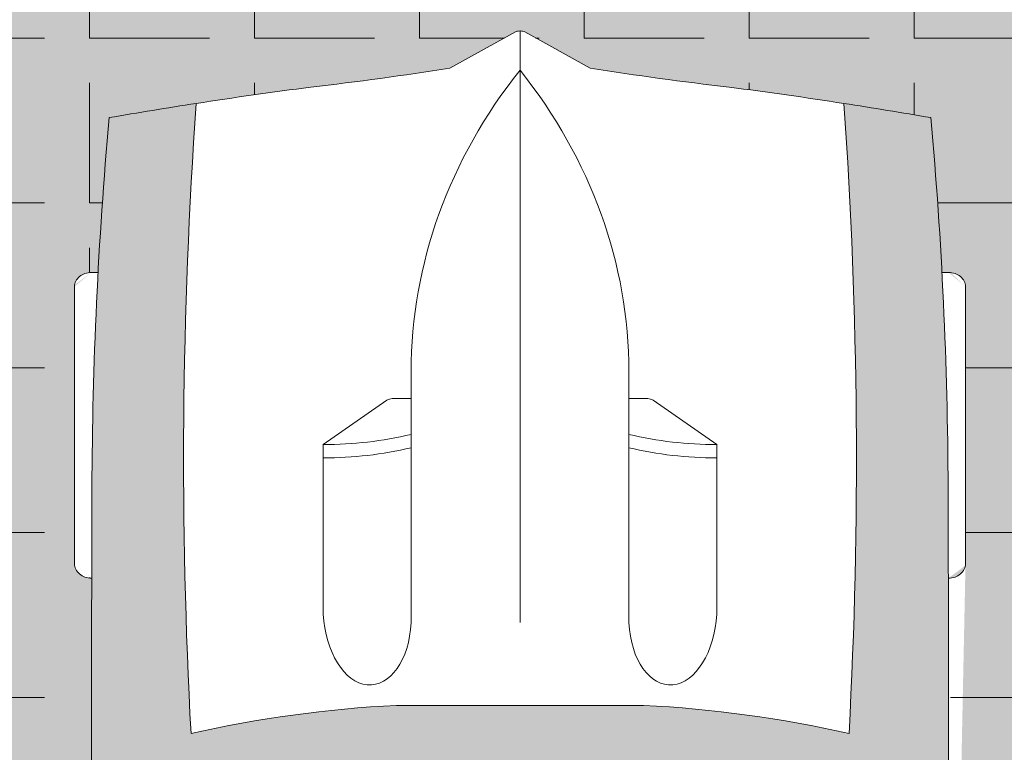
# Model space of a CAD drawing. Units: millimetres. Extents: x 1166 to 16630, y -7192 to 2820.
# Tile 4 of 8: x 5842 to 7051, y -3952 to -3052. Entities that reach past the tile are written whole.
import ezdxf

# ---------------------------------------------------------------- set-up
doc = ezdxf.new("R2010")
doc.units = ezdxf.units.MM
doc.layers.add('A-FLOR-FNSH-PATT', color=254, linetype='Continuous', lineweight=13, true_color=0xfeeab9)
doc.layers.add('C-PKNG-VEHI-PATT', color=18, linetype='Continuous', lineweight=13, true_color=0x000000)
doc.layers.add('A-FLOR-PATT', color=8, linetype='Continuous', lineweight=13)
doc.layers.add('C-PKNG-VEHI', color=8, linetype='Continuous', lineweight=18)

# ---------------------------------------------------------------- blocks, each defined once
blk = doc.blocks.new('*U6')
for p, q in [((46.55368679439944, 38.88847654282876), (22.35054758993934, 38.88847654282876)), ((21.10406751471477, 37.40863046792069), (21.10406751471477, 36.83230215753705)), ((47.80016686962392, 37.39011648242055), (47.80016686962392, 37.40863046792069)), ((32.26591480791686, 11.62530558863241), (36.12873726252356, 17.16961494239206)), ((36.12873726252356, 17.16961494239206), (50.93891189819171, 17.16961494239206)), ((32.12291633764599, 9.505833383620029), (32.12291633764599, 11.15369945057711)), ((58.9167604809788, -10.77488335095668), (58.9167604809788, 10.77488335095617)), ((29.77279020470884, 9.505833383620029), (51.68362801571248, 9.505833383620029)), ((3.266462181856987, 6.128290093440767), (0.1022408397004821, 0.4060708604429806)), ((-4.43e-14, -2.558e-13), (51.68362801571248, -2.558e-13)), ((0.1022408397004821, -0.4060708604432933), (3.266462181856987, -6.128290093441194)), ((29.77279020470884, -9.50583338362054), (51.68362801571248, -9.50583338362054)), ((32.12291633764599, -9.50583338362054), (32.12291633764599, -11.15369945057762)), ((32.26591480791686, -11.62530558863292), (36.12873726252356, -17.16961494239257)), ((36.12873726252356, -17.16961494239257), (50.93891189819171, -17.16961494239257)), ((21.10406751471477, -37.4086304679212), (21.10406751471477, -36.83230215753756)), ((47.80016686962392, -37.39011648242107), (47.80016686962392, -37.4086304679212)), ((46.55368679439944, -38.88847654282927), (22.35054758993934, -38.88847654282927))]:
    blk.add_line(p, q)
for centre, major_axis, ratio, start_param, end_param in [((22.35054758993934, 37.40863046792072), (2.08e-14, -1.479846074908118), 0.842303869543976, 3.141592653589776, 4.712388980384677), ((46.55368679439944, 37.40863046792072), (2.2e-14, 1.479846074908118), 0.8423038695439758, -1.570796326794884, 1.73e-14), ((41.19115208863305, -490.8631038926156), (1.294e-13, 528.2339998381949), 0.8423038695439741, 0.0028100083536837, 0.0755983031096952), ((64.48199294511879, -10555.61767587835), (1.907644e-10, 10593.02630634627), 0.842303869543847, -0.0133969486112073, 0.0027970409639888), ((266.0300214172791, -27.52442688366631), (1.966072e-10, 313.3077612809058), 0.8423038695435284, 1.367075990158062, 1.391760499156098), ((37.47375371777758, -593.9621830607928), (6.21e-14, -623.32820996736), 0.8423038695439826, 3.09604606856106, 3.200911180495224), ((134.4003789125686, 5.387441675477674), (4.276e-13, -89.7774543484738), 0.84230386954398, 4.44948196380473, 4.652344057257214), ((259.1750197310735, -27.52442688366614), (1.506617e-10, -305.3028914627677), 0.8423038695443789, 4.528606069860317, 4.561837674556238), ((-204.4946649195746, 52.39684969293512), (4.12053e-11, -250.9602162198571), 0.8423038695441164, 1.385369446298923, 1.434372047871027), ((13.03653510440275, 17.00972444508943), (1.2303e-12, 27.41599049210566), 0.8423038695439277, 4.435146050259648, 4.718221029521873), ((14.20086229321332, 17.00972444508943), (1.2303e-12, 27.41599049210566), 0.8423038695439277, 4.435146050259648, 4.718221029521873), ((50.7902773840875, 13.33772416300607), (6.340077547122382, -0.356608581037027), 0.6038335755719145, -1.39555193967809, 1.581314658479915), ((32.74615637525823, 11.15369945057713), (1.313e-13, 0.7399230374541176), 0.8423038695439091, 0.8797135699495516, 1.570796326795045), ((29.77279020470884, -46.66302566589627), (5.12e-14, 56.16885904951626), 0.842303869543976, 7e-16, 0.5903187773915901), ((0.6232400376122422, -1.421e-13), (1e-16, -0.7399230374541245), 0.842303869543842, 4.131459131953847, 5.293318828815531), ((29.77279020470884, 46.66302566589578), (4.004e-13, 56.16885904951626), 0.8423038695439734, 2.55127387619821, 3.141592653589801), ((-204.4946649195746, -52.39684969293552), (4.02945e-11, 250.9602162198562), 0.8423038695441192, -1.43437204787103, -1.385369446298926), ((13.03653510440275, -17.00972444508983), (1.2568e-12, -27.41599049210552), 0.8423038695439318, 1.564964277657711, 1.848039256919935), ((14.20086229321332, -17.00972444508983), (1.2568e-12, -27.41599049210552), 0.8423038695439318, 1.564964277657711, 1.848039256919935), ((32.74615637525823, -11.1536994505777), (1.3e-13, -0.7399230374541176), 0.8423038695439093, 4.712388980384541, 5.403471737230034), ((134.4003789125684, -5.387441675478584), (4.2949e-12, -89.77745434847827), 0.8423038695439354, -1.510751403667474, -1.307889310215002), ((259.1750197310694, 27.52442688365929), (1.08535e-11, 305.3028914629043), 0.8423038695439974, 1.721347632622872, 1.754579237318777), ((266.0300214172791, 27.52442688366566), (8.75241e-11, 313.3077612806533), 0.8423038695441819, 1.749832154434603, 1.774516663432659), ((37.47375371777847, 593.9621830607904), (1.1693e-12, -623.3282099673584), 0.8423038695439528, -0.0593185269054384, 0.0455465850287298), ((41.19115208863322, 490.8631038926152), (1.37757e-11, -528.2339998381949), 0.8423038695440652, -0.0755983031097181, -0.0028100083537155), ((64.48199294495228, 10555.61767590795), (6.117947e-10, 10593.02630637587), 0.8423038695458146, 3.138795612625926, 3.154989602201039), ((22.35054758993934, -37.40863046792117), (2.2e-14, 1.479846074908118), 0.8423038695439758, 1.570796326794908, 3.14159265358981), ((46.55368679439944, -37.40863046792117), (2.08e-14, -1.479846074908118), 0.842303869543976, -1.69e-14, 1.570796326794884)]:
    blk.add_ellipse(centre, major_axis=major_axis, ratio=ratio, start_param=start_param, end_param=end_param)
at = {"extrusion": (0, 0, -1)}
blk.add_ellipse((50.7902773840875, -13.33772416300655), major_axis=(6.340077547122382, 0.3566085810370246), ratio=0.6038335755719145, start_param=-1.39555193967809, end_param=1.581314658479915, dxfattribs=at)

msp = doc.modelspace()

# ---------------------------------------------------------------- hatches: boundary and pattern name
at = {"layer": 'A-FLOR-FNSH-PATT', "transparency": 33554590}
h = msp.add_hatch(color=256, dxfattribs=at)
h.dxf.hatch_style = 1
h.paths.add_polyline_path([(5309.614992693758, -2642.53776490782), (5309.614992693758, -6304.141088113749), (7725.939441137629, -6304.141088113749), (7725.939441137629, -5672.53776490782), (7725.939441137629, -2642.53776490782)])
edge = h.paths.add_edge_path(flags=16)
edge.add_ellipse((-448.9724108440159, -3645.429588524165), major_axis=(-7430.722679011307, 2.05049e-10), ratio=0.8423038695440578, start_angle=182.1799503136468, end_angle=183.6504275857006, ccw=False)
edge.add_line((6974.17381326888, -3362.862478220109), (6984.715647929133, -3362.862478220109))
edge.add_ellipse((6982.28108362224, -3380.396843230207), major_axis=(-20.81714882728829, 5.19e-13), ratio=0.842303869543992, start_angle=180.0000000000014, end_angle=270.0000000000014, ccw=False)
edge.add_line((7003.098232449528, -3380.396843230198), (7003.098232449528, -3722.915565549822))
edge.add_ellipse((6982.28108362224, -3720.864922613471), major_axis=(20.81714882728829, 5.097e-13), ratio=0.842303869543992, start_angle=269.9999999999985, end_angle=359.9999999999986, ccw=False)
edge.add_ellipse((-142030.922985108, -3973.064272051784), major_axis=(149013.2040687302, 7.3876543e-09), ratio=0.8423038695454406, start_angle=-0.3838667787953227, end_angle=0.09022908859151357, ccw=False)
edge.add_line((6977.567346638728, -4971.397229994678), (6984.470063297348, -4971.397229994678))
edge.add_ellipse((6982.28108362224, -4988.931595004776), major_axis=(20.81714882728829, 5.4695e-12), ratio=0.84230386954397, start_angle=-1.5006662579253316e-11, end_angle=89.99999999998488, ccw=False)
edge.add_line((7003.098232449528, -4988.931595004766), (7003.098232449527, -5331.243460438734))
edge.add_ellipse((6982.281083622239, -5329.399674388036), major_axis=(-20.81714882728829, 1.0505e-12), ratio=0.84230386954397, start_angle=90.0000000000029, end_angle=180.000000000003, ccw=False)
edge.add_line((6982.281083622243, -5346.934039398132), (6973.353954790083, -5346.934039398132))
edge.add_ellipse((-142030.922985108, -3973.064272051784), major_axis=(149013.2040687302, 7.3876543e-09), ratio=0.8423038695454406, start_angle=-0.6186431963221253, end_angle=-0.5282714718208013, ccw=False)
edge.add_ellipse((6960.189207408767, -5606.902802775503), major_axis=(-31.22572324093233, 2.0889e-12), ratio=0.8423038695439425, start_angle=179.3717627838109, end_angle=248.4647566010108, ccw=False)
edge.add_ellipse((-142041.331559525, -3973.064272085929), major_axis=(-149045.3717863939, 4.64621177404e-05), ratio=0.8423038661083152, start_angle=179.3534459208122, end_angle=179.3717628016453, ccw=False)
edge.add_ellipse((6916.869834512962, -5654.054118847628), major_axis=(-73.80201542105252, 3.6097e-12), ratio=0.8423038695439748, start_angle=90.00000000006492, end_angle=179.353445902922, ccw=False)
edge.add_line((6916.869834513031, -5716.217842016925), (5995.230132669023, -5716.217842016909))
edge.add_ellipse((5995.230132669163, -5654.054118847574), major_axis=(73.80201542109666, 3.978e-13), ratio=0.8423038695439887, start_angle=180.6465540970575, end_angle=269.9999999998622, ccw=False)
edge.add_ellipse((154953.4315273228, -3973.06427200764), major_axis=(-149045.3717871212, 2.2898328512e-06), ratio=0.8423038697262194, start_angle=0.6282372171232851, end_angle=0.6465540979564253, ccw=False)
edge.add_ellipse((5951.910759773294, -5606.902802775455), major_axis=(31.22572324094488, 4.9039e-12), ratio=0.842303869543988, start_angle=111.53524350401449, end_angle=180.6282372161637, ccw=False)
edge.add_ellipse((154943.0229527065, -3973.064272049507), major_axis=(-149013.2040691466, 7.4869171e-09), ratio=0.8423038695459824, start_angle=0.528271471820176, end_angle=0.6465540970638131, ccw=False)
edge.add_line((5938.746012391977, -5346.934039398132), (5927.384319252956, -5346.934039398132))
edge.add_ellipse((5929.818883559845, -5329.399674388033), major_axis=(20.8171488272892, 3.11e-13), ratio=0.8423038695440205, start_angle=179.9999999999992, end_angle=269.9999999999962, ccw=False)
edge.add_line((5909.001734732555, -5329.399674388034), (5909.001734732554, -4986.88095206843))
edge.add_ellipse((5929.818883559843, -4988.931595004776), major_axis=(-20.8171488272892, 3.063e-13), ratio=0.8423038695440205, start_angle=-89.99999999999608, end_angle=7.958078640513122e-13, ccw=False)
edge.add_line((5929.818883559843, -4971.397229994676), (5934.53262054336, -4971.397229994676))
edge.add_ellipse((154943.0229527065, -3973.064272049507), major_axis=(-149013.2040691466, 7.4869171e-09), ratio=0.8423038695459824, start_angle=-0.09022908859031986, end_angle=0.38386677879520903, ccw=False)
edge.add_ellipse((5929.818883559843, -3720.864922613471), major_axis=(-20.8171488272892, 1.5867e-12), ratio=0.8423038695439331, start_angle=4.376943252282217e-12, end_angle=90.00000000000438, ccw=False)
edge.add_line((5909.001734732555, -3720.864922613478), (5909.001734732555, -3378.346200293855))
edge.add_ellipse((5929.818883559843, -3380.396843230207), major_axis=(20.8171488272892, 9.396e-13), ratio=0.8423038695439548, start_angle=89.99999999999739, end_angle=179.9999999999975, ccw=False)
edge.add_line((5929.818883559843, -3362.862478220109), (5937.926153913206, -3362.862478220109))
edge.add_ellipse((13361.0723780261, -3645.42958852417), major_axis=(7430.722679011307, 7.96527e-11), ratio=0.8423038695440075, start_angle=176.3495724143003, end_angle=177.8200496863542, ccw=False)
edge.add_ellipse((6843.238962592569, -6808.26137511002), major_axis=(4407.332901654202, 4.993684e-10), ratio=0.8423038695438785, start_angle=102.12596555227748, end_angle=103.7805289894913, ccw=False)
edge.add_ellipse((6843.238962592481, -6711.831352601092), major_axis=(4294.727564406183, 8.108409e-10), ratio=0.8423038695438188, start_angle=100.20953899713243, end_angle=102.4446272934332, ccw=False)
edge.add_ellipse((5718.978043047074, -189.3416182050969), major_axis=(-3530.283493235897, 2.29487e-11), ratio=0.8423038695439934, start_angle=99.25656600720184, end_angle=102.5549326441376)
edge.add_line((6369.842688727707, -3111.939026631001), (6452.046781461999, -3066.482546539763))
edge.add_ellipse((6456.049983591043, -3074.756545497792), major_axis=(-10.40857441364578, 1.5838e-12), ratio=0.8423038695437935, start_angle=270.0000000000206, end_angle=307.9331304598557, ccw=False)
edge.add_ellipse((6456.049983591043, -3074.756545497792), major_axis=(-10.40857441364578, 1.5838e-12), ratio=0.8423038695437935, start_angle=232.06686954016618, end_angle=270.0000000000206, ccw=False)
edge.add_line((6461.762224667734, -3067.427595530816), (6542.257278454378, -3111.939026631002))
edge.add_ellipse((7193.121924135012, -189.3416182050969), major_axis=(3530.283493235459, 5.426614e-10), ratio=0.842303869544094, start_angle=257.4450673558539, end_angle=260.7434339927895)
edge.add_ellipse((6068.861004589511, -6711.831352601148), major_axis=(4294.72756440461, 7.517164e-10), ratio=0.8423038695441345, start_angle=77.55537270654469, end_angle=79.79046100284552, ccw=False)
edge.add_ellipse((6068.86100458951, -6808.26137511002), major_axis=(-4407.332901654327, 6.637773e-10), ratio=0.842303869543856, start_angle=256.2194710105107, end_angle=257.8740344477245, ccw=False)
edge = h.paths.add_edge_path(flags=0)
edge.add_ellipse((5799.636342679871, -3484.80630294614), major_axis=(790.1331889300527, 2.1537e-12), ratio=0.8423038695439757, start_angle=-2.2737367544323206e-13, end_angle=29.43856959797921, ccw=False)
edge.add_line((6589.769531609924, -3484.806302946152), (6589.769531609924, -3517.865771969153))
edge.add_line((6589.769531609924, -3517.865771969153), (6615.396946753699, -3517.865771969153))
edge.add_ellipse((6612.950235160742, -3526.632954474201), major_axis=(10.40857441364348, 1.5653e-12), ratio=0.8423038695440233, start_angle=45.51978911742219, end_angle=89.99999999999147, ccw=False)
edge.add_line((6619.58436781158, -3519.877346340421), (6697.576744801804, -3574.216072032502))
edge.add_line((6697.576744801804, -3574.216072032502), (6697.576744801804, -3782.552340767745))
edge.add_ellipse((6643.673138205864, -3780.461483581003), major_axis=(5.016450041930374, 89.18653102701357), ratio=0.6038335755719256, start_angle=106.34259195429391, end_angle=270.99798572497, ccw=False)
edge.add_line((6589.769531609924, -3793.028339937766), (6589.769531609924, -3484.806302946153))
edge.add_ellipse((5799.636342679871, -3484.80630294614), major_axis=(790.1331889300527, 2.1537e-12), ratio=0.8423038695439757, start_angle=-2.143e-13, end_angle=29.43856959797918)
edge.add_ellipse((7112.463624502211, -3484.80630294614), major_axis=(-790.1331889300524, 7.9434e-12), ratio=0.8423038695439707, start_angle=-29.43856959797882, end_angle=5.465e-13)
edge.add_line((6322.330435572158, -3484.806302946151), (6322.330435572158, -3793.028339937766))
edge.add_ellipse((6268.426828976219, -3780.461483581003), major_axis=(-5.016450041930374, 89.18653102701357), ratio=0.6038335755719256, start_angle=89.00201427502998, end_angle=253.6574080457062, ccw=False)
edge.add_line((6214.523222380278, -3782.552340767737), (6214.523222380279, -3574.216072032502))
edge.add_line((6214.523222380279, -3574.216072032502), (6294.400928520307, -3518.563802793423))
edge.add_ellipse((6299.149732021341, -3526.632954474201), major_axis=(10.4085744136453, 3.381e-13), ratio=0.8423038695438764, start_angle=89.9999999999983, end_angle=134.4802108825654, ccw=False)
edge.add_line((6299.149732021338, -3517.865771969152), (6322.330435572158, -3517.865771969152))
edge.add_line((6322.330435572158, -3517.865771969152), (6322.330435572158, -3484.806302946154))
edge.add_ellipse((7112.463624502211, -3484.80630294614), major_axis=(-790.1331889300524, 7.9434e-12), ratio=0.8423038695439707, start_angle=-29.438569597978812, end_angle=6.252776074688882e-13, ccw=False)
edge = h.paths.add_edge_path(flags=0)
edge.add_line((6899.672020630411, -4051.112638739672), (6868.937058315451, -4281.473694083312))
edge.add_ellipse((6495.430033257824, -5170.362894493258), major_axis=(1119.455420763322, 3.0514e-12), ratio=0.8423038695439744, start_angle=67.20808512240981, end_angle=85.12993040286408)
edge.add_line((6575.564661792019, -4229.860228440724), (6336.53530539007, -4229.860228440724))
edge.add_ellipse((6416.669933924288, -5170.362894493482), major_axis=(1119.455420763633, 5.82337e-11), ratio=0.842303869543943, start_angle=94.87006959713275, end_angle=112.7919148775836)
edge.add_line((6043.162908866626, -4281.473694083309), (6012.427946551666, -4051.112638739666))
edge.add_ellipse((6380.264280565288, -4969.144446445703), major_axis=(1150.303461305961, 5.9583e-11), ratio=0.8423038695439412, start_angle=94.27742096305099, end_angle=111.83495379670521, ccw=False)
edge.add_line((6307.939299228742, -4002.156437400477), (6604.160667953341, -4002.156437400477))
edge.add_ellipse((6531.835686616772, -4969.144446445682), major_axis=(-1150.303461305901, 2.25473e-11), ratio=0.8423038695439672, start_angle=248.1650462032914, end_angle=265.72257903694555, ccw=False)
edge = h.paths.add_edge_path(flags=0)
edge.add_ellipse((-142030.9229855244, -3973.064272050007), major_axis=(-148992.3869203194, 2.076209e-10), ratio=0.842303869544003, start_angle=179.6222358060902, end_angle=179.9444056865007, ccw=False)
edge.add_line((6956.899516505626, -4955.389335168179), (6903.06848209712, -4744.029778632651))
edge.add_ellipse((-45118.92430422086, -4413.460367112857), major_axis=(52023.47313689829, 7.771381e-10), ratio=0.842303869543516, start_angle=-0.3640763488911976, end_angle=0.1208973690317991)
edge.add_line((6904.3855953652, -4303.688047353878), (6961.365076797346, -4117.63210307358))
edge = h.paths.add_edge_path(flags=0)
edge.add_line((5950.734890384741, -4117.632103073563), (6007.714371816899, -4303.688047353918))
edge.add_ellipse((58031.02427140294, -4413.460367113082), major_axis=(-52023.47313689826, 1.3200601e-09), ratio=0.8423038695497072, start_angle=-0.1208973690315197, end_angle=0.364076348891516)
edge.add_line((6009.031485084967, -4744.029778632643), (5955.200450676423, -4955.389335168309))
edge.add_ellipse((154943.0229527063, -3973.064272050686), major_axis=(-148992.3869203192, 3.28274152e-08), ratio=0.8423038695536886, start_angle=0.05559431351167632, end_angle=0.3777641939223031, ccw=False)
edge = h.paths.add_edge_path(flags=0)
edge.add_line((6868.937058315452, -5013.198477251068), (6868.937058315452, -5277.993200767081))
edge.add_ellipse((6456.049983591043, -3571.079447459644), major_axis=(2068.11644385622, 7.9333e-12), ratio=0.8423038695439821, start_angle=256.4018653097692, end_angle=283.59813469023027, ccw=False)
edge.add_line((6043.16290886663, -5277.993200767081), (6043.16290886663, -5013.198477251068))
edge.add_ellipse((6456.049983591043, -3306.284723943631), major_axis=(2068.116443856253, 3.3411e-12), ratio=0.8423038695439679, start_angle=256.4018653097692, end_angle=283.5981346902304)
edge = h.paths.add_edge_path(flags=0)
edge.add_ellipse((6827.302760660877, -5415.313265203762), major_axis=(-41.63429765457658, 1.038e-12), ratio=0.842303869543992, start_angle=180.0000000000014, end_angle=270.0000000000014, ccw=False)
edge.add_line((6868.937058315454, -5415.313265203762), (6868.937058315454, -5689.12284886784))
edge.add_line((6868.937058315454, -5689.12284886784), (6043.162908866631, -5689.122848867824))
edge.add_line((6043.162908866631, -5689.122848867824), (6043.16290886663, -5415.313265203758))
edge.add_ellipse((6084.797206521206, -5415.313265203759), major_axis=(-41.63429765457658, 3.4138e-12), ratio=0.842303869543992, start_angle=-89.99999999999523, end_angle=4.718003765447065e-12, ccw=False)
edge.add_line((6084.797206521207, -5380.244535183563), (6827.302760660879, -5380.244535183566))
h.paths.add_polyline_path([(3455.939441137629, -522.53776490782), (1955.939441137629, -522.53776490782), (1955.939441137629, -2522.53776490782), (3455.939441137629, -2522.53776490782), (3455.939441137628, -2456.640093510054), (2713.439441137629, -2456.640093510054), (2713.43944113763, -2423.827593510054), (2714.157558370035, -2423.827593510054, -0.398552660000795), (3455.939441137629, -1706.6775944476)])
h.paths.add_polyline_path([(2617.666699633915, -1084.404517764245, -0.1328909081885223), (2584.2707950462, -1084.404517500826, -0.5013167773008519), (2505.064916213601, -782.9330743979599), (2537.033121160981, -687.0284595558127), (2489.081652205778, -687.0284595558132), (2489.081652205778, -711.0041940334158), (2441.130183250573, -711.0041940334158), (2441.130183250573, -695.0203710483474), (2473.097829220709, -695.0203710483474), (2473.097829220709, -687.0284595558132), (2433.13827175804, -687.0284595558132), (2433.138271758038, -559.1578756752674), (2768.79855444447, -559.1578756752674), (2768.798554444471, -687.0284595558132), (2664.903705041528, -687.0284595558132), (2696.870765296628, -782.9296403211174, -0.5013234908365807)], flags=16)
h.paths.add_polyline_path([(2627.246667254758, -1063.015793855155, -0.2150037826753064), (2574.690827957319, -1063.015793301825, -0.4800796505537303), (2537.033991046725, -782.9313974662227), (2664.904416594217, -782.9313974662227, -0.4800795019660876)], flags=0)
h.paths.add_polyline_path([(2736.830905816404, -671.0446365707452), (2465.105920386107, -671.0446365707452, -0.5000001164022092), (2449.122094743107, -655.0608109277463), (2449.122094743107, -591.1255243033341, -0.5000001164022404), (2465.105920386111, -575.1416986603361), (2736.830905816402, -575.1416986603361, -0.5000001164023353), (2752.814731459403, -591.1255243033406), (2752.814731459403, -655.0608109277468, -0.50000011640211)], flags=0)
h.paths.add_polyline_path([(5931.781743219382, -6111.826019846759), (7070.309755611069, -6111.826019846759), (7070.309755611069, -5852.301891921869), (5931.781743219382, -5852.301891921869)], flags=24)
h.paths.add_polyline_path([(2102.335631979146, -1543.656328414819), (3007.075088498303, -1543.656328414819), (3007.075088498303, -1283.961010431932), (2102.335631979146, -1283.961010431932)], flags=24)
at = {"layer": 'A-FLOR-PATT', "transparency": 33554564}
h = msp.add_hatch(dxfattribs=at)
h.set_pattern_fill('ANGLE', color=256, scale=29)
h.set_pattern_definition([(0, (-8657.519420588213, -11987.85165359825), (0, 202.565), [147.32, -55.24499999999999]), (90, (-8657.519420588213, -11987.85165359825), (-202.565, 1.24e-14), [147.32, -55.24499999999999])])
h.paths.add_polyline_path([(7725.939441137629, -2642.53776490782), (5309.614992693758, -2642.53776490782), (5309.614992693758, -6304.141088113749), (7725.939441137629, -6304.141088113749), (7725.939441137629, -5672.53776490782)])
edge = h.paths.add_edge_path(flags=16)
edge.add_ellipse((-142030.922985108, -3973.064272051784), major_axis=(149013.2040687302, 7.3876543e-09), ratio=0.8423038695454406, start_angle=-0.3838667787953227, end_angle=0.09022908859151357, ccw=False)
edge.add_ellipse((6982.28108362224, -4988.931595004776), major_axis=(20.81714882728829, 5.4695e-12), ratio=0.84230386954397, start_angle=-1.5006662579253316e-11, end_angle=89.99999999998488, ccw=False)
edge.add_line((7003.098232449528, -4988.931595004773), (7003.098232449527, -5329.399674388036))
edge.add_ellipse((6982.281083622239, -5329.399674388036), major_axis=(-20.81714882728829, 1.0505e-12), ratio=0.84230386954397, start_angle=90.0000000000029, end_angle=180.000000000003, ccw=False)
edge.add_line((6982.281083622241, -5346.934039398132), (6973.353954790083, -5346.934039398132))
edge.add_ellipse((-142030.922985108, -3973.064272051784), major_axis=(149013.2040687302, 7.3876543e-09), ratio=0.8423038695454406, start_angle=-0.6186431963221253, end_angle=-0.5282714718208013, ccw=False)
edge.add_ellipse((6960.189207408767, -5606.902802775503), major_axis=(-31.22572324093233, 2.0889e-12), ratio=0.8423038695439425, start_angle=179.3717627838109, end_angle=248.4647566010108, ccw=False)
edge.add_ellipse((-142041.331559525, -3973.064272085929), major_axis=(-149045.3717863939, 4.64621177404e-05), ratio=0.8423038661083152, start_angle=179.3534459208122, end_angle=179.3717628016453, ccw=False)
edge.add_ellipse((6916.869834512962, -5654.054118847628), major_axis=(-73.80201542105252, 3.6097e-12), ratio=0.8423038695439748, start_angle=90.00000000006492, end_angle=179.353445902922, ccw=False)
edge.add_line((6916.869834513029, -5716.217842016925), (5995.230132669016, -5716.217842016909))
edge.add_ellipse((5995.230132669163, -5654.054118847574), major_axis=(73.80201542109666, 3.978e-13), ratio=0.8423038695439887, start_angle=180.6465540970575, end_angle=269.9999999998622, ccw=False)
edge.add_ellipse((154953.4315273228, -3973.06427200764), major_axis=(-149045.3717871212, 2.2898328512e-06), ratio=0.8423038697262194, start_angle=0.6282372171232851, end_angle=0.6465540979564253, ccw=False)
edge.add_ellipse((5951.910759773294, -5606.902802775455), major_axis=(31.22572324094488, 4.9039e-12), ratio=0.842303869543988, start_angle=111.53524350401449, end_angle=180.6282372161637, ccw=False)
edge.add_ellipse((154943.0229527065, -3973.064272049507), major_axis=(-149013.2040691466, 7.4869171e-09), ratio=0.8423038695459824, start_angle=0.528271471820176, end_angle=0.6465540970638131, ccw=False)
edge.add_line((5938.746012391977, -5346.934039398132), (5929.818883559843, -5346.934039398132))
edge.add_ellipse((5929.818883559845, -5329.399674388033), major_axis=(20.8171488272892, 3.11e-13), ratio=0.8423038695440205, start_angle=179.9999999999992, end_angle=269.9999999999962, ccw=False)
edge.add_line((5909.001734732555, -5329.399674388033), (5909.001734732554, -4988.931595004778))
edge.add_ellipse((5929.818883559843, -4988.931595004776), major_axis=(-20.8171488272892, 3.063e-13), ratio=0.8423038695440205, start_angle=-89.99999999999608, end_angle=7.958078640513122e-13, ccw=False)
edge.add_ellipse((154943.0229527065, -3973.064272049507), major_axis=(-149013.2040691466, 7.4869171e-09), ratio=0.8423038695459824, start_angle=-0.09022908859031986, end_angle=0.38386677879520903, ccw=False)
edge.add_ellipse((5929.818883559843, -3720.864922613471), major_axis=(-20.8171488272892, 1.5867e-12), ratio=0.8423038695439331, start_angle=4.376943252282217e-12, end_angle=90.00000000000438, ccw=False)
edge.add_line((5909.001734732555, -3720.864922613472), (5909.001734732555, -3380.396843230204))
edge.add_ellipse((5929.818883559843, -3380.396843230207), major_axis=(20.8171488272892, 9.396e-13), ratio=0.8423038695439548, start_angle=89.99999999999739, end_angle=179.9999999999975, ccw=False)
edge.add_line((5929.818883559843, -3362.862478220109), (5937.926153913207, -3362.862478220109))
edge.add_ellipse((13361.0723780261, -3645.42958852417), major_axis=(7430.722679011307, 7.96527e-11), ratio=0.8423038695440075, start_angle=176.3495724143003, end_angle=177.8200496863542, ccw=False)
edge.add_ellipse((6843.238962592569, -6808.26137511002), major_axis=(4407.332901654202, 4.993684e-10), ratio=0.8423038695438785, start_angle=102.12596555227748, end_angle=103.7805289894913, ccw=False)
edge.add_ellipse((6843.238962592481, -6711.831352601092), major_axis=(4294.727564406183, 8.108409e-10), ratio=0.8423038695438188, start_angle=100.20953899713243, end_angle=102.4446272934332, ccw=False)
edge.add_ellipse((5718.978043047074, -189.3416182050969), major_axis=(-3530.283493235897, 2.29487e-11), ratio=0.8423038695439934, start_angle=99.25656600720184, end_angle=102.5549326441376)
edge.add_line((6369.842688727707, -3111.939026631), (6453.505541262713, -3065.675894661087))
edge.add_ellipse((6456.049983591043, -3074.756545497792), major_axis=(-10.40857441364578, 1.5838e-12), ratio=0.8423038695437935, start_angle=232.06686954016618, end_angle=270.0000000000206, ccw=False)
edge.add_line((6460.053185720086, -3066.482546539763), (6542.257278454378, -3111.939026631002))
edge.add_ellipse((7193.121924135012, -189.3416182050969), major_axis=(3530.283493235459, 5.426614e-10), ratio=0.842303869544094, start_angle=257.4450673558539, end_angle=260.7434339927895)
edge.add_ellipse((6068.861004589511, -6711.831352601148), major_axis=(4294.72756440461, 7.517164e-10), ratio=0.8423038695441345, start_angle=77.55537270654469, end_angle=79.79046100284552, ccw=False)
edge.add_ellipse((6068.86100458951, -6808.26137511002), major_axis=(-4407.332901654327, 6.637773e-10), ratio=0.842303869543856, start_angle=256.2194710105107, end_angle=257.8740344477245, ccw=False)
edge.add_ellipse((-448.9724108440159, -3645.429588524165), major_axis=(-7430.722679011307, 2.05049e-10), ratio=0.8423038695440578, start_angle=182.1799503136468, end_angle=183.6504275857006, ccw=False)
edge.add_line((6974.17381326888, -3362.862478220109), (6982.28108362224, -3362.862478220109))
edge.add_ellipse((6982.28108362224, -3380.396843230207), major_axis=(-20.81714882728829, 5.19e-13), ratio=0.842303869543992, start_angle=180.0000000000014, end_angle=270.0000000000014, ccw=False)
edge.add_line((7003.098232449528, -3380.396843230204), (7003.098232449528, -3720.864922613474))
edge.add_ellipse((6982.28108362224, -3720.864922613471), major_axis=(20.81714882728829, 5.097e-13), ratio=0.842303869543992, start_angle=269.9999999999985, end_angle=359.9999999999986, ccw=False)
edge = h.paths.add_edge_path(flags=0)
edge.add_ellipse((-142030.9229855244, -3973.064272050007), major_axis=(-148992.3869203194, 2.076209e-10), ratio=0.842303869544003, start_angle=179.6222358060902, end_angle=179.9444056865007, ccw=False)
edge.add_line((6956.899516505626, -4955.389335168179), (6903.06848209712, -4744.029778632651))
edge.add_ellipse((-45118.92430422086, -4413.460367112857), major_axis=(52023.47313689829, 7.771381e-10), ratio=0.842303869543516, start_angle=-0.3640763488911976, end_angle=0.1208973690317991)
edge.add_line((6904.3855953652, -4303.688047353878), (6961.365076797346, -4117.632103073563))
edge = h.paths.add_edge_path(flags=0)
edge.add_line((6899.672020630411, -4051.112638739673), (6868.937058315451, -4281.473694083312))
edge.add_ellipse((6495.430033257824, -5170.362894493258), major_axis=(1119.455420763322, 3.0514e-12), ratio=0.8423038695439744, start_angle=67.20808512240981, end_angle=85.12993040286408)
edge.add_line((6575.564661792022, -4229.860228440724), (6336.535305390071, -4229.860228440724))
edge.add_ellipse((6416.669933924288, -5170.362894493482), major_axis=(1119.455420763633, 5.82337e-11), ratio=0.842303869543943, start_angle=94.87006959713275, end_angle=112.7919148775836)
edge.add_line((6043.162908866626, -4281.473694083308), (6012.427946551666, -4051.112638739666))
edge.add_ellipse((6380.264280565288, -4969.144446445703), major_axis=(1150.303461305961, 5.9583e-11), ratio=0.8423038695439412, start_angle=94.27742096305099, end_angle=111.83495379670521, ccw=False)
edge.add_line((6307.939299228742, -4002.156437400477), (6604.16066795334, -4002.156437400477))
edge.add_ellipse((6531.835686616772, -4969.144446445682), major_axis=(-1150.303461305901, 2.25473e-11), ratio=0.8423038695439672, start_angle=248.1650462032914, end_angle=265.72257903694555, ccw=False)
edge = h.paths.add_edge_path(flags=0)
edge.add_ellipse((6643.673138205864, -3780.461483581003), major_axis=(5.016450041930374, 89.18653102701357), ratio=0.6038335755719256, start_angle=106.34259195429391, end_angle=270.99798572497, ccw=False)
edge.add_line((6589.769531609924, -3793.028339937766), (6589.769531609924, -3484.806302946154))
edge.add_ellipse((5799.636342679871, -3484.80630294614), major_axis=(790.1331889300527, 2.1537e-12), ratio=0.8423038695439757, start_angle=-2.143e-13, end_angle=29.43856959797918)
edge.add_ellipse((7112.463624502211, -3484.80630294614), major_axis=(-790.1331889300524, 7.9434e-12), ratio=0.8423038695439707, start_angle=-29.43856959797882, end_angle=5.465e-13)
edge.add_line((6322.330435572158, -3484.806302946151), (6322.330435572158, -3793.028339937766))
edge.add_ellipse((6268.426828976219, -3780.461483581003), major_axis=(-5.016450041930374, 89.18653102701357), ratio=0.6038335755719256, start_angle=89.00201427502998, end_angle=253.6574080457062, ccw=False)
edge.add_line((6214.523222380278, -3782.552340767735), (6214.523222380279, -3574.216072032502))
edge.add_line((6214.523222380279, -3574.216072032502), (6295.402812213822, -3517.865771969152))
edge.add_line((6295.402812213822, -3517.865771969152), (6322.330435572158, -3517.865771969152))
edge.add_line((6322.330435572158, -3517.865771969152), (6322.330435572158, -3484.806302946154))
edge.add_ellipse((7112.463624502211, -3484.80630294614), major_axis=(-790.1331889300524, 7.9434e-12), ratio=0.8423038695439707, start_angle=-29.438569597978812, end_angle=6.252776074688882e-13, ccw=False)
edge.add_ellipse((5799.636342679871, -3484.80630294614), major_axis=(790.1331889300527, 2.1537e-12), ratio=0.8423038695439757, start_angle=-2.2737367544323206e-13, end_angle=29.43856959797921, ccw=False)
edge.add_line((6589.769531609924, -3484.806302946153), (6589.769531609924, -3517.865771969153))
edge.add_line((6589.769531609924, -3517.865771969153), (6616.697154968261, -3517.865771969153))
edge.add_line((6616.697154968261, -3517.865771969153), (6697.576744801804, -3574.216072032502))
edge.add_line((6697.576744801804, -3574.216072032502), (6697.576744801804, -3782.552340767746))
edge = h.paths.add_edge_path(flags=0)
edge.add_line((6868.937058315452, -5013.198477251068), (6868.937058315452, -5277.993200767081))
edge.add_ellipse((6456.049983591043, -3571.079447459644), major_axis=(2068.11644385622, 7.9333e-12), ratio=0.8423038695439821, start_angle=256.4018653097692, end_angle=283.59813469023027, ccw=False)
edge.add_line((6043.16290886663, -5277.993200767081), (6043.16290886663, -5013.198477251067))
edge.add_ellipse((6456.049983591043, -3306.284723943631), major_axis=(2068.116443856253, 3.3411e-12), ratio=0.8423038695439679, start_angle=256.4018653097692, end_angle=283.5981346902304)
edge = h.paths.add_edge_path(flags=0)
edge.add_ellipse((58031.02427140294, -4413.460367113082), major_axis=(-52023.47313689826, 1.3200601e-09), ratio=0.8423038695497072, start_angle=-0.1208973690315197, end_angle=0.364076348891516)
edge.add_line((6009.031485084967, -4744.029778632643), (5955.200450676423, -4955.389335168309))
edge.add_ellipse((154943.0229527063, -3973.064272050686), major_axis=(-148992.3869203192, 3.28274152e-08), ratio=0.8423038695536886, start_angle=0.05559431351167632, end_angle=0.3777641939223031, ccw=False)
edge.add_line((5950.734890384742, -4117.632103073569), (6007.714371816899, -4303.688047353918))
edge = h.paths.add_edge_path(flags=0)
edge.add_ellipse((6827.302760660877, -5415.313265203762), major_axis=(-41.63429765457658, 1.038e-12), ratio=0.842303869543992, start_angle=180.0000000000014, end_angle=270.0000000000014, ccw=False)
edge.add_line((6868.937058315454, -5415.313265203762), (6868.937058315454, -5689.12284886784))
edge.add_line((6868.937058315454, -5689.12284886784), (6043.162908866631, -5689.122848867824))
edge.add_line((6043.162908866631, -5689.122848867824), (6043.16290886663, -5415.31326520376))
edge.add_ellipse((6084.797206521206, -5415.313265203759), major_axis=(-41.63429765457658, 3.4138e-12), ratio=0.842303869543992, start_angle=-89.99999999999523, end_angle=4.718003765447065e-12, ccw=False)
edge.add_line((6084.797206521206, -5380.244535183563), (6827.302760660877, -5380.244535183566))
at = {"layer": 'C-PKNG-VEHI-PATT'}
h = msp.add_hatch(color=256, dxfattribs=at)
h.dxf.hatch_style = 1
edge = h.paths.add_edge_path()
edge.add_ellipse((-142030.922985108, -3973.064272051784), major_axis=(149013.2040687302, 7.3876543e-09), ratio=0.8423038695454406, start_angle=-0.3838667787953527, end_angle=0.0902290885914815)
edge.add_ellipse((-142030.922985108, -3973.064272051784), major_axis=(149013.2040687302, 7.3876543e-09), ratio=0.8423038695454406, start_angle=0.0902290885914815, end_angle=0.1349865768554186)
edge.add_ellipse((-448.9724108440159, -3645.429588524165), major_axis=(-7430.722679011307, 2.05049e-10), ratio=0.8423038695440578, start_angle=180.1356123904399, end_angle=182.1799503136467)
edge.add_ellipse((-448.9724108440159, -3645.429588524165), major_axis=(-7430.722679011307, 2.05049e-10), ratio=0.8423038695440578, start_angle=182.1799503136467, end_angle=183.6504275857006)
edge.add_ellipse((6068.86100458951, -6808.26137511002), major_axis=(-4407.332901654327, 6.637773e-10), ratio=0.842303869543856, start_angle=256.2194710105107, end_angle=257.8740344477245)
edge.add_ellipse((-1899.27789287437, -3593.136558560746), major_axis=(-8768.422834748915, 4.33705e-11), ratio=0.8423038695439387, start_angle=177.8014594340451, end_angle=182.8637146078378, ccw=False)
edge.add_ellipse((6531.835686616759, -4956.613487829934), major_axis=(1262.90879855413, 2.05481e-11), ratio=0.8423038695439913, start_angle=72.28004677724863, end_angle=85.91758930884843)
edge.add_line((6607.621389642485, -3894.777567489213), (6304.478577539601, -3894.777567489213))
edge.add_ellipse((6380.264280565318, -4956.613487829931), major_axis=(1262.908798554214, 5.95268e-11), ratio=0.8423038695439325, start_angle=94.08241069114744, end_angle=107.7199532227473)
edge.add_ellipse((14811.37786005643, -3593.136558560761), major_axis=(8768.422834748895, 2.19537e-11), ratio=0.8423038695438954, start_angle=177.1362853921622, end_angle=182.1985405659549, ccw=False)
edge.add_ellipse((6843.238962592569, -6808.26137511002), major_axis=(4407.332901654202, 4.993684e-10), ratio=0.8423038695438785, start_angle=102.1259655522775, end_angle=103.7805289894913)
edge.add_ellipse((13361.0723780261, -3645.42958852417), major_axis=(7430.722679011307, 7.96527e-11), ratio=0.8423038695440075, start_angle=176.3495724143003, end_angle=177.8200496863541)
edge.add_ellipse((13361.0723780261, -3645.42958852417), major_axis=(7430.722679011307, 7.96527e-11), ratio=0.8423038695440075, start_angle=177.8200496863541, end_angle=179.8643876095608)
edge.add_ellipse((154943.0229527065, -3973.064272049507), major_axis=(-149013.2040691466, 7.4869171e-09), ratio=0.8423038695459824, start_angle=-0.1349865768541338, end_angle=-0.0902290885903158)
edge.add_ellipse((154943.0229527065, -3973.064272049507), major_axis=(-149013.2040691466, 7.4869171e-09), ratio=0.8423038695459824, start_angle=-0.0902290885903158, end_angle=0.3838667787951928)
edge.add_ellipse((154943.0229527065, -3973.064272049507), major_axis=(-149013.2040691466, 7.4869171e-09), ratio=0.8423038695459824, start_angle=0.3838667787951928, end_angle=0.5282714718202328)
edge.add_ellipse((154943.0229527065, -3973.064272049507), major_axis=(-149013.2040691466, 7.4869171e-09), ratio=0.8423038695459824, start_angle=0.5282714718202328, end_angle=0.6465540970638061)
edge.add_ellipse((5984.821558255466, -5654.054118847628), major_axis=(41.63429765457481, 1.0657e-12), ratio=0.8423038695440057, start_angle=180.6465540970899, end_angle=269.9999999999108)
edge.add_line((5984.821558255388, -5689.122848867822), (6043.162908866631, -5689.122848867825))
edge.add_line((6043.162908866631, -5689.122848867825), (6043.16290886663, -5411.211979331063))
edge.add_ellipse((6084.797206521206, -5415.313265203759), major_axis=(-41.63429765457658, 3.4138e-12), ratio=0.842303869543992, start_angle=-89.99999999999523, end_angle=4.718003765447065e-12, ccw=False)
edge.add_line((6084.797206521205, -5380.244535183563), (6832.171889274661, -5380.244535183566))
edge.add_ellipse((6827.302760660877, -5415.313265203762), major_axis=(-41.63429765457658, 1.038e-12), ratio=0.842303869543992, start_angle=180.0000000000014, end_angle=270.0000000000014, ccw=False)
edge.add_line((6868.937058315454, -5415.313265203762), (6868.937058315454, -5689.12284886784))
edge.add_line((6868.937058315454, -5689.12284886784), (6927.278408926672, -5689.122848867841))
edge.add_ellipse((6927.278408926624, -5654.054118847645), major_axis=(-41.63429765457638, 9.732e-13), ratio=0.8423038695439738, start_angle=90.00000000008009, end_angle=179.3534459029312)
edge.add_ellipse((-142030.922985108, -3973.064272051784), major_axis=(149013.2040687302, 7.3876543e-09), ratio=0.8423038695454406, start_angle=-0.646554097064762, end_angle=-0.6186431963220466)
edge.add_ellipse((-142030.922985108, -3973.064272051784), major_axis=(149013.2040687302, 7.3876543e-09), ratio=0.8423038695454406, start_angle=-0.6186431963220466, end_angle=-0.5282714718207955)
edge.add_ellipse((-142030.922985108, -3973.064272051784), major_axis=(149013.2040687302, 7.3876543e-09), ratio=0.8423038695454406, start_angle=-0.5282714718207955, end_angle=-0.3838667787953527)
edge = h.paths.add_edge_path(flags=16)
edge.add_ellipse((6416.669933924288, -5170.362894493482), major_axis=(1119.455420763633, 5.82337e-11), ratio=0.842303869543943, start_angle=94.87006959713275, end_angle=112.7919148775836)
edge.add_line((6043.162908866626, -4281.473694083309), (6012.427946551666, -4051.112638739666))
edge.add_ellipse((6380.264280565288, -4969.144446445703), major_axis=(1150.303461305961, 5.9583e-11), ratio=0.8423038695439412, start_angle=94.27742096305099, end_angle=111.83495379670521, ccw=False)
edge.add_line((6307.93929922874, -4002.156437400477), (6604.16066795334, -4002.156437400477))
edge.add_ellipse((6531.835686616772, -4969.144446445682), major_axis=(-1150.303461305901, 2.25473e-11), ratio=0.8423038695439672, start_angle=248.1650462032914, end_angle=265.72257903694555, ccw=False)
edge.add_line((6899.672020630411, -4051.112638739672), (6868.937058315451, -4281.473694083312))
edge.add_ellipse((6495.430033257824, -5170.362894493258), major_axis=(1119.455420763322, 3.0514e-12), ratio=0.8423038695439744, start_angle=67.20808512240981, end_angle=85.12993040286408)
edge.add_line((6575.564661792022, -4229.860228440724), (6336.535305390071, -4229.860228440724))
edge = h.paths.add_edge_path(flags=16)
edge.add_ellipse((58031.02427140294, -4413.460367113082), major_axis=(-52023.47313689826, 1.3200601e-09), ratio=0.8423038695497072, start_angle=-0.1208973690315197, end_angle=0.364076348891516)
edge.add_line((6009.031485084967, -4744.029778632643), (5955.200450676423, -4955.389335168309))
edge.add_ellipse((154943.0229527063, -3973.064272050686), major_axis=(-148992.3869203192, 3.28274152e-08), ratio=0.8423038695536886, start_angle=0.05559431351167632, end_angle=0.3777641939223031, ccw=False)
edge.add_line((5950.734890384742, -4117.632103073569), (6007.714371816899, -4303.688047353918))
edge = h.paths.add_edge_path(flags=16)
edge.add_line((6904.3855953652, -4303.688047353878), (6961.365076797346, -4117.63210307357))
edge.add_ellipse((-142030.9229855244, -3973.064272050007), major_axis=(-148992.3869203194, 2.076209e-10), ratio=0.842303869544003, start_angle=179.6222358060902, end_angle=179.9444056865007, ccw=False)
edge.add_line((6956.899516505626, -4955.38933516818), (6903.06848209712, -4744.029778632651))
edge.add_ellipse((-45118.92430422086, -4413.460367112857), major_axis=(52023.47313689829, 7.771381e-10), ratio=0.842303869543516, start_angle=-0.3640763488911976, end_angle=0.1208973690317991)
edge = h.paths.add_edge_path(flags=16)
edge.add_ellipse((6456.049983591043, -3306.284723943631), major_axis=(2068.116443856253, 3.3411e-12), ratio=0.8423038695439679, start_angle=256.4018653097692, end_angle=283.5981346902304)
edge.add_line((6868.937058315452, -5013.198477251068), (6868.937058315452, -5277.993200767081))
edge.add_ellipse((6456.049983591043, -3571.079447459644), major_axis=(2068.11644385622, 7.9333e-12), ratio=0.8423038695439821, start_angle=256.4018653097692, end_angle=283.59813469023027, ccw=False)
edge.add_line((6043.16290886663, -5277.993200767081), (6043.16290886663, -5013.198477251067))

# ---------------------------------------------------------------- block references
at = {"layer": 'C-PKNG-VEHI', "xscale": 14.06710412674579, "yscale": 14.06710412674579, "zscale": 14.06710412674579, "rotation": 270}
msp.add_blockref('*U6', (6456.049983591045, -3065.989362992743), dxfattribs=at)

doc.saveas('drawing.dxf')
